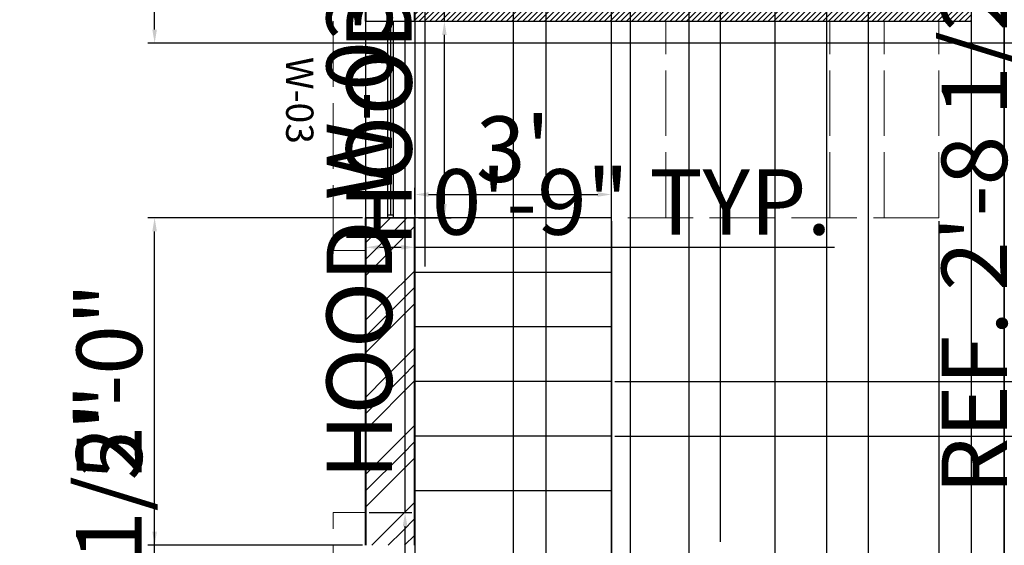
# Model space of a CAD drawing. Units: inches. Extents: x 2386 to 3029, y 792 to 1465.
# Tile 5 of 12: x 2408 to 2588, y 1044 to 1140. Entities that reach past the tile are written whole.
import ezdxf

# ---------------------------------------------------------------- set-up
doc = ezdxf.new("R2010")
doc.units = ezdxf.units.IN
doc.linetypes.add('ACAD_ISO02W100', pattern=[15, 12, -3])
for name, color, linetype, lineweight in [('A-DIMS', 1, 'Continuous', 18), ('A-STAIR', 7, 'Continuous', 25), ('A-STAIR-OVHD', 7, 'ACAD_ISO02W100', 18), ('A-TEXT', 4, 'Continuous', 25), ('A-WALL-EXT', 7, 'Continuous', 40), ('A-WALL-INT', 9, 'Continuous', 30), ('A-WALL-PATT', 9, 'Continuous', 13), ('A-WINDOW', 4, 'Continuous', 25), ('A-WINDOW-OVHD', 4, 'ACAD_ISO02W100', 18)]:
    doc.layers.add(name, color=color, linetype=linetype, lineweight=lineweight)
doc.styles.get("Standard").update_dxf_attribs({"font": 'arial.ttf'})
doc.dimstyles.new('ISO-25', dxfattribs={"dimtxt": 12, "dimasz": 2.5, "dimexe": 1.25, "dimexo": 0.625, "dimtad": 1, "dimlunit": 4, "dimtxsty": 'Standard', "dimcen": 2.5, "dimadec": 0, "dimazin": 0, "dimtfac": 1, "dimtmove": 0, "dimatfit": 3, "dimfxl": 1, "dimarcsym": 0})

# ---------------------------------------------------------------- blocks, each defined once
blk = doc.blocks.new('*D18')
at = {"layer": 'A-DIMS', "color": 0, "lineweight": -2, "transparency": 16777216}
for p, q in [((2480.19, 1104.57), (2480.19, 1109.47)), ((2482.69, 1108.22), (2513.69, 1108.22)), ((2516.19, 1104.57), (2516.19, 1109.47))]:
    blk.add_line(p, q, dxfattribs=at)
at = {"layer": 'A-DIMS', "color": 0, "transparency": 16777216}
for points in [[(2482.69, 1108.64), (2482.69, 1107.81), (2480.19, 1108.22)], [(2513.69, 1108.64), (2513.69, 1107.81), (2516.19, 1108.22)]]:
    blk.add_solid(points, dxfattribs=at)
at = {"layer": 'Defpoints', "color": 0, "transparency": 16777216}
for p in [(2516.19, 1108.22), (2480.19, 1103.95), (2516.19, 1103.95)]:
    blk.add_point(p, dxfattribs=at)
at = {"layer": 'A-DIMS', "color": 0, "transparency": 16777216, "insert": (2498.19, 1114.98), "char_height": 12, "attachment_point": 5}
blk.add_mtext("3'", dxfattribs=at)
blk = doc.blocks.new('WINDOW-36IN')
for p, q in [((0, 0), (0, 36)), ((4, 36), (4, 0)), ((4, 35.5), (5, 35.5)), ((4.5, 35.5), (4.5, 0.5)), ((5, 36), (5, 0)), ((9, 36), (9, 0)), ((5, 0.5), (4, 0.5))]:
    blk.add_line(p, q)
blk = doc.blocks.new('WINDOW-HOOD-36IN')
for p, q in [((0, 0), (0, 48)), ((0, 48), (6, 48)), ((6, 0), (0, 0))]:
    blk.add_line(p, q)
blk = doc.blocks.new('*D38')
at = {"layer": 'A-DIMS', "color": 0, "lineweight": -2, "transparency": 16777216}
for p, q in [((2471.82, 1342.95), (2483.24, 1342.95)), ((2481.99, 1340.45), (2481.99, 1273.45)), ((2471.82, 1270.95), (2483.24, 1270.95)), ((2481.99, 1270.95), (2481.99, 1095.04))]:
    blk.add_line(p, q, dxfattribs=at)
at = {"layer": 'A-DIMS', "color": 0, "transparency": 16777216}
for points in [[(2481.57, 1340.45), (2482.41, 1340.45), (2481.99, 1342.95)], [(2481.57, 1273.45), (2482.41, 1273.45), (2481.99, 1270.95)]]:
    blk.add_solid(points, dxfattribs=at)
at = {"layer": 'Defpoints', "color": 0, "transparency": 16777216}
for p in [(2471.19, 1342.95), (2471.19, 1270.95), (2481.99, 1270.95)]:
    blk.add_point(p, dxfattribs=at)
at = {"layer": 'A-DIMS', "color": 0, "transparency": 16777216, "insert": (2475.16, 1181.74), "char_height": 12, "attachment_point": 5, "rotation": 90}
blk.add_mtext('HOOD W-01 6\'-0" TYP.', dxfattribs=at)
blk = doc.blocks.new('*D44')
at = {"layer": 'A-DIMS', "color": 0, "lineweight": -2, "transparency": 16777216}
for p, q in [((2485.59, 1139.95), (2485.59, 1262.04)), ((2480.82, 1139.95), (2486.84, 1139.95)), ((2485.59, 1106.45), (2485.59, 1137.45)), ((2480.82, 1103.95), (2486.84, 1103.95))]:
    blk.add_line(p, q, dxfattribs=at)
at = {"layer": 'A-DIMS', "color": 0, "transparency": 16777216}
for points in [[(2485.17, 1137.45), (2486.01, 1137.45), (2485.59, 1139.95)], [(2485.17, 1106.45), (2486.01, 1106.45), (2485.59, 1103.95)]]:
    blk.add_solid(points, dxfattribs=at)
at = {"layer": 'Defpoints', "color": 0, "transparency": 16777216}
for p in [(2480.19, 1139.95), (2485.59, 1139.95), (2480.19, 1103.95)]:
    blk.add_point(p, dxfattribs=at)
at = {"layer": 'A-DIMS', "color": 0, "transparency": 16777216, "insert": (2478.83, 1202.25), "char_height": 12, "attachment_point": 5, "rotation": 90}
blk.add_mtext('W-03 3\'-0" TYP.', dxfattribs=at)
blk = doc.blocks.new('*D45')
at = {"layer": 'A-DIMS', "color": 0, "lineweight": -2, "transparency": 16777216}
for p, q in [((2471.19, 1103.32), (2471.19, 1097.3)), ((2480.19, 1103.32), (2480.19, 1097.3)), ((2473.69, 1098.55), (2477.69, 1098.55)), ((2480.19, 1098.55), (2557.09, 1098.55))]:
    blk.add_line(p, q, dxfattribs=at)
at = {"layer": 'A-DIMS', "color": 0, "transparency": 16777216}
for points in [[(2473.69, 1098.96), (2473.69, 1098.13), (2471.19, 1098.55)], [(2477.69, 1098.96), (2477.69, 1098.13), (2480.19, 1098.55)]]:
    blk.add_solid(points, dxfattribs=at)
at = {"layer": 'Defpoints', "color": 0, "transparency": 16777216}
for p in [(2471.19, 1103.95), (2480.19, 1103.95), (2480.19, 1098.55)]:
    blk.add_point(p, dxfattribs=at)
at = {"layer": 'A-DIMS', "color": 0, "transparency": 16777216, "insert": (2519.89, 1105.3), "char_height": 12, "attachment_point": 5}
blk.add_mtext('0\'-9" TYP.', dxfattribs=at)
blk = doc.blocks.new('*D46')
at = {"layer": 'A-DIMS', "color": 0, "lineweight": -2, "transparency": 16777216}
for p, q in [((2478.39, 1049.95), (2478.39, 1225.86)), ((2471.82, 1049.95), (2479.64, 1049.95)), ((2478.39, 1004.45), (2478.39, 1047.45)), ((2471.82, 1001.95), (2479.64, 1001.95))]:
    blk.add_line(p, q, dxfattribs=at)
at = {"layer": 'A-DIMS', "color": 0, "transparency": 16777216}
for points in [[(2477.97, 1047.45), (2478.81, 1047.45), (2478.39, 1049.95)], [(2477.97, 1004.45), (2478.81, 1004.45), (2478.39, 1001.95)]]:
    blk.add_solid(points, dxfattribs=at)
at = {"layer": 'Defpoints', "color": 0, "transparency": 16777216}
for p in [(2471.19, 1049.95), (2478.39, 1049.95), (2471.19, 1001.95)]:
    blk.add_point(p, dxfattribs=at)
at = {"layer": 'A-DIMS', "color": 0, "transparency": 16777216, "insert": (2471.55, 1139.15), "char_height": 12, "attachment_point": 5, "rotation": 90}
blk.add_mtext('HOOD W-03 4\'-0" TYP.', dxfattribs=at)
blk = doc.blocks.new('*D52')
at = {"layer": 'A-DIMS', "color": 0, "lineweight": -2, "transparency": 16777216}
for p, q in [((2595.33, 1229.95), (2589.83, 1229.95)), ((2591.08, 1227.45), (2591.08, 1199.96)), ((2595.33, 1197.46), (2589.83, 1197.46)), ((2591.08, 1197.46), (2591.08, 1050.38))]:
    blk.add_line(p, q, dxfattribs=at)
at = {"layer": 'A-DIMS', "color": 0, "transparency": 16777216}
for points in [[(2590.67, 1227.45), (2591.5, 1227.45), (2591.08, 1229.95)], [(2590.67, 1199.96), (2591.5, 1199.96), (2591.08, 1197.46)]]:
    blk.add_solid(points, dxfattribs=at)
at = {"layer": 'Defpoints', "color": 0, "transparency": 16777216}
for p in [(2595.96, 1229.95), (2591.08, 1197.46), (2595.96, 1197.46)]:
    blk.add_point(p, dxfattribs=at)
at = {"layer": 'A-DIMS', "color": 0, "transparency": 16777216, "insert": (2584.25, 1122.67), "char_height": 12, "attachment_point": 5, "rotation": 90}
blk.add_mtext('REF. 2\'-8 1/2" TYP.', dxfattribs=at)
blk = doc.blocks.new('*D57')
at = {"layer": 'A-DIMS', "color": 0, "lineweight": -2, "transparency": 16777216}
for p, q in [((2546.19, 1008.57), (2546.19, 1427.9)), ((2582.19, 1008.57), (2582.19, 1427.9)), ((2548.69, 1426.65), (2579.69, 1426.65))]:
    blk.add_line(p, q, dxfattribs=at)
at = {"layer": 'A-DIMS', "color": 0, "transparency": 16777216}
for points in [[(2548.69, 1427.06), (2548.69, 1426.23), (2546.19, 1426.65)], [(2579.69, 1427.06), (2579.69, 1426.23), (2582.19, 1426.65)]]:
    blk.add_solid(points, dxfattribs=at)
at = {"layer": 'Defpoints', "color": 0, "transparency": 16777216}
for p in [(2582.19, 1426.65), (2546.19, 1007.95), (2582.19, 1007.95)]:
    blk.add_point(p, dxfattribs=at)
at = {"layer": 'A-DIMS', "color": 0, "transparency": 16777216, "insert": (2564.19, 1433.4), "char_height": 12, "attachment_point": 5}
blk.add_mtext('3\'-0"', dxfattribs=at)
blk = doc.blocks.new('*D62')
at = {"layer": 'A-DIMS', "color": 0, "lineweight": -2, "transparency": 16777216}
for p, q in [((2432.49, 1007.95), (2432.49, 1072.04)), ((2470.57, 1007.95), (2431.24, 1007.95)), ((2432.49, 955.95), (2432.49, 1005.45)), ((2470.57, 953.45), (2431.24, 953.45))]:
    blk.add_line(p, q, dxfattribs=at)
at = {"layer": 'A-DIMS', "color": 0, "transparency": 16777216}
for points in [[(2432.07, 1005.45), (2432.91, 1005.45), (2432.49, 1007.95)], [(2432.07, 955.95), (2432.91, 955.95), (2432.49, 953.45)]]:
    blk.add_solid(points, dxfattribs=at)
at = {"layer": 'Defpoints', "color": 0, "transparency": 16777216}
for p in [(2432.49, 1007.95), (2471.19, 1007.95), (2471.19, 953.45)]:
    blk.add_point(p, dxfattribs=at)
at = {"layer": 'A-DIMS', "color": 0, "transparency": 16777216, "insert": (2425.66, 1041.24), "char_height": 12, "attachment_point": 5, "rotation": 90}
blk.add_mtext('4\'-6 1/2"', dxfattribs=at)
blk = doc.blocks.new('*D63')
at = {"layer": 'A-DIMS', "color": 0, "lineweight": -2, "transparency": 16777216}
for p, q in [((2470.57, 1103.95), (2431.24, 1103.95)), ((2432.49, 1046.45), (2432.49, 1101.45)), ((2470.57, 1043.95), (2431.24, 1043.95))]:
    blk.add_line(p, q, dxfattribs=at)
at = {"layer": 'A-DIMS', "color": 0, "transparency": 16777216}
for points in [[(2432.07, 1101.45), (2432.91, 1101.45), (2432.49, 1103.95)], [(2432.07, 1046.45), (2432.91, 1046.45), (2432.49, 1043.95)]]:
    blk.add_solid(points, dxfattribs=at)
at = {"layer": 'Defpoints', "color": 0, "transparency": 16777216}
for p in [(2432.49, 1103.95), (2471.19, 1103.95), (2471.19, 1043.95)]:
    blk.add_point(p, dxfattribs=at)
at = {"layer": 'A-DIMS', "color": 0, "transparency": 16777216, "insert": (2425.74, 1073.95), "char_height": 12, "attachment_point": 5, "rotation": 90}
blk.add_mtext('5\'-0"', dxfattribs=at)
blk = doc.blocks.new('*D73')
at = {"layer": 'A-DIMS', "color": 0, "lineweight": -2, "transparency": 16777216}
for p, q in [((2519.68, 889.97), (2519.68, 1427.9)), ((2555.68, 889.97), (2555.68, 1427.9)), ((2522.18, 1426.65), (2553.18, 1426.65))]:
    blk.add_line(p, q, dxfattribs=at)
at = {"layer": 'A-DIMS', "color": 0, "transparency": 16777216}
for points in [[(2522.18, 1427.06), (2522.18, 1426.23), (2519.68, 1426.65)], [(2553.18, 1427.06), (2553.18, 1426.23), (2555.68, 1426.65)]]:
    blk.add_solid(points, dxfattribs=at)
at = {"layer": 'Defpoints', "color": 0, "transparency": 16777216}
for p in [(2555.68, 1426.65), (2519.68, 889.35), (2555.68, 889.35)]:
    blk.add_point(p, dxfattribs=at)
at = {"layer": 'A-DIMS', "color": 0, "transparency": 16777216, "insert": (2537.68, 1433.4), "char_height": 12, "attachment_point": 5}
blk.add_mtext('3\'-0"', dxfattribs=at)
blk = doc.blocks.new('*D76')
at = {"layer": 'A-DIMS', "color": 0, "lineweight": -2, "transparency": 16777216}
for p, q in [((2480.19, 1174.77), (2480.19, 808)), ((2498.19, 1174.77), (2498.19, 808)), ((2482.69, 809.25), (2495.69, 809.25)), ((2498.19, 809.25), (2532.71, 809.25))]:
    blk.add_line(p, q, dxfattribs=at)
at = {"layer": 'A-DIMS', "color": 0, "transparency": 16777216}
for points in [[(2482.69, 809.66), (2482.69, 808.83), (2480.19, 809.25)], [(2495.69, 809.66), (2495.69, 808.83), (2498.19, 809.25)]]:
    blk.add_solid(points, dxfattribs=at)
at = {"layer": 'Defpoints', "color": 0, "transparency": 16777216}
for p in [(2480.19, 1175.39), (2498.19, 1175.39), (2498.19, 809.25)]:
    blk.add_point(p, dxfattribs=at)
at = {"layer": 'A-DIMS', "color": 0, "transparency": 16777216, "insert": (2516.7, 816), "char_height": 12, "attachment_point": 5}
blk.add_mtext('1\'-6"', dxfattribs=at)
blk = doc.blocks.new('*D77')
at = {"layer": 'A-DIMS', "color": 0, "lineweight": -2, "transparency": 16777216}
for p, q in [((2516.19, 1103.32), (2516.19, 808)), ((2576.19, 1103.32), (2576.19, 808)), ((2518.69, 809.25), (2573.69, 809.25))]:
    blk.add_line(p, q, dxfattribs=at)
at = {"layer": 'A-DIMS', "color": 0, "transparency": 16777216}
for points in [[(2518.69, 809.66), (2518.69, 808.83), (2516.19, 809.25)], [(2573.69, 809.66), (2573.69, 808.83), (2576.19, 809.25)]]:
    blk.add_solid(points, dxfattribs=at)
at = {"layer": 'Defpoints', "color": 0, "transparency": 16777216}
for p in [(2516.19, 1103.95), (2576.19, 1103.95), (2576.19, 809.25)]:
    blk.add_point(p, dxfattribs=at)
at = {"layer": 'A-DIMS', "color": 0, "transparency": 16777216, "insert": (2546.19, 816), "char_height": 12, "attachment_point": 5}
blk.add_mtext('5\'-0"', dxfattribs=at)
blk = doc.blocks.new('*D78')
at = {"layer": 'A-DIMS', "color": 0, "lineweight": -2, "transparency": 16777216}
for p, q in [((2516.19, 1054.57), (2516.19, 1427.9)), ((2536.19, 1044.57), (2536.19, 1427.9)), ((2518.69, 1426.65), (2533.69, 1426.65)), ((2536.19, 1426.65), (2570.71, 1426.65))]:
    blk.add_line(p, q, dxfattribs=at)
at = {"layer": 'A-DIMS', "color": 0, "transparency": 16777216}
for points in [[(2518.69, 1427.06), (2518.69, 1426.23), (2516.19, 1426.65)], [(2533.69, 1427.06), (2533.69, 1426.23), (2536.19, 1426.65)]]:
    blk.add_solid(points, dxfattribs=at)
at = {"layer": 'Defpoints', "color": 0, "transparency": 16777216}
for p in [(2536.19, 1426.65), (2516.19, 1053.95), (2536.19, 1043.95)]:
    blk.add_point(p, dxfattribs=at)
at = {"layer": 'A-DIMS', "color": 0, "transparency": 16777216, "insert": (2554.7, 1433.4), "char_height": 12, "attachment_point": 5}
blk.add_mtext('1\'-8"', dxfattribs=at)
blk = doc.blocks.new('*D79')
at = {"layer": 'A-DIMS', "color": 0, "lineweight": -2, "transparency": 16777216}
for p, q in [((2929.89, 1073.95), (2929.89, 1118.92)), ((2516.82, 1073.95), (2931.14, 1073.95)), ((2929.89, 1066.45), (2929.89, 1071.45)), ((2516.82, 1063.95), (2931.14, 1063.95))]:
    blk.add_line(p, q, dxfattribs=at)
at = {"layer": 'A-DIMS', "color": 0, "transparency": 16777216}
for points in [[(2929.47, 1071.45), (2930.31, 1071.45), (2929.89, 1073.95)], [(2929.47, 1066.45), (2930.31, 1066.45), (2929.89, 1063.95)]]:
    blk.add_solid(points, dxfattribs=at)
at = {"layer": 'Defpoints', "color": 0, "transparency": 16777216}
for p in [(2516.19, 1073.95), (2929.89, 1073.95), (2516.19, 1063.95)]:
    blk.add_point(p, dxfattribs=at)
at = {"layer": 'A-DIMS', "color": 0, "transparency": 16777216, "insert": (2923.14, 1097.68), "char_height": 12, "attachment_point": 5, "rotation": 90}
blk.add_mtext('0\'-10"', dxfattribs=at)
blk = doc.blocks.new('*D81')
at = {"layer": 'A-DIMS', "color": 0, "lineweight": -2, "transparency": 16777216}
for p, q in [((2432.49, 1153.95), (2432.49, 1188.47)), ((2809.57, 1153.95), (2431.24, 1153.95)), ((2432.49, 1138.45), (2432.49, 1151.45)), ((2809.57, 1135.95), (2431.24, 1135.95))]:
    blk.add_line(p, q, dxfattribs=at)
at = {"layer": 'A-DIMS', "color": 0, "transparency": 16777216}
for points in [[(2432.07, 1151.45), (2432.91, 1151.45), (2432.49, 1153.95)], [(2432.07, 1138.45), (2432.91, 1138.45), (2432.49, 1135.95)]]:
    blk.add_solid(points, dxfattribs=at)
at = {"layer": 'Defpoints', "color": 0, "transparency": 16777216}
for p in [(2432.49, 1153.95), (2810.19, 1153.95), (2810.19, 1135.95)]:
    blk.add_point(p, dxfattribs=at)
at = {"layer": 'A-DIMS', "color": 0, "transparency": 16777216, "insert": (2425.74, 1172.46), "char_height": 12, "attachment_point": 5, "rotation": 90}
blk.add_mtext('1\'-6"', dxfattribs=at)
blk = doc.blocks.new('*D94')
at = {"layer": 'A-DIMS', "color": 0, "lineweight": -2, "transparency": 16777216}
for p, q in [((2504.19, 1205.32), (2504.19, 808)), ((2588.19, 1205.32), (2588.19, 808)), ((2506.69, 809.25), (2585.69, 809.25))]:
    blk.add_line(p, q, dxfattribs=at)
at = {"layer": 'A-DIMS', "color": 0, "transparency": 16777216}
for points in [[(2506.69, 809.66), (2506.69, 808.83), (2504.19, 809.25)], [(2585.69, 809.66), (2585.69, 808.83), (2588.19, 809.25)]]:
    blk.add_solid(points, dxfattribs=at)
at = {"layer": 'Defpoints', "color": 0, "transparency": 16777216}
for p in [(2504.19, 1205.95), (2588.19, 1205.95), (2588.19, 809.25)]:
    blk.add_point(p, dxfattribs=at)
at = {"layer": 'A-DIMS', "color": 0, "transparency": 16777216, "insert": (2546.19, 816), "char_height": 12, "attachment_point": 5}
blk.add_mtext('7\'-0"', dxfattribs=at)
blk = doc.blocks.new('*D96')
at = {"layer": 'A-DIMS', "color": 0, "lineweight": -2, "transparency": 16777216}
for p, q in [((2516.19, 893.57), (2516.19, 1427.9)), ((2588.19, 893.57), (2588.19, 1427.9)), ((2518.69, 1426.65), (2585.69, 1426.65))]:
    blk.add_line(p, q, dxfattribs=at)
at = {"layer": 'A-DIMS', "color": 0, "transparency": 16777216}
for points in [[(2518.69, 1427.06), (2518.69, 1426.23), (2516.19, 1426.65)], [(2585.69, 1427.06), (2585.69, 1426.23), (2588.19, 1426.65)]]:
    blk.add_solid(points, dxfattribs=at)
at = {"layer": 'Defpoints', "color": 0, "transparency": 16777216}
for p in [(2588.19, 1426.65), (2516.19, 892.95), (2588.19, 892.95)]:
    blk.add_point(p, dxfattribs=at)
at = {"layer": 'A-DIMS', "color": 0, "transparency": 16777216, "insert": (2552.19, 1433.4), "char_height": 12, "attachment_point": 5}
blk.add_mtext('6\'-0"', dxfattribs=at)
blk = doc.blocks.new('*D99')
at = {"layer": 'A-DIMS', "color": 0, "lineweight": -2, "transparency": 16777216}
for p, q in [((2530.41, 1210.29), (2530.41, 808)), ((2563.26, 1210.63), (2563.26, 808)), ((2532.91, 809.25), (2560.76, 809.25)), ((2563.26, 809.25), (2599.11, 809.25))]:
    blk.add_line(p, q, dxfattribs=at)
at = {"layer": 'A-DIMS', "color": 0, "transparency": 16777216}
for points in [[(2532.91, 809.66), (2532.91, 808.83), (2530.41, 809.25)], [(2560.76, 809.66), (2560.76, 808.83), (2563.26, 809.25)]]:
    blk.add_solid(points, dxfattribs=at)
at = {"layer": 'Defpoints', "color": 0, "transparency": 16777216}
for p in [(2530.41, 1210.91), (2563.26, 1211.26), (2563.26, 809.25)]:
    blk.add_point(p, dxfattribs=at)
at = {"layer": 'A-DIMS', "color": 0, "transparency": 16777216, "insert": (2582.43, 816), "char_height": 12, "attachment_point": 5}
blk.add_mtext('2\'-9"', dxfattribs=at)

msp = doc.modelspace()

# ---------------------------------------------------------------- hatches: boundary and pattern name
at = {"layer": 'A-WALL-PATT'}
h = msp.add_hatch(dxfattribs=at)
h.set_pattern_fill('GOST_GROUND', color=256)
h.paths.add_polyline_path([(2480.19, 1276.948), (2471.19, 1276.948), (2471.19, 1211.948), (2480.19, 1211.948)])
h.paths.add_polyline_path([(2480.19, 1378.948), (2510.19, 1378.948), (2510.19, 1378.969), (2523.779, 1378.969), (2580.602, 1378.959), (2580.602, 1378.969), (2594.19, 1378.969), (2642.19, 1378.948), (2642.19, 1387.948), (2471.19, 1387.948), (2471.19, 1336.948), (2480.19, 1336.948)])
h.paths.add_polyline_path([(2891.19, 1387.948), (2666.19, 1387.948), (2666.19, 1378.948), (2882.19, 1378.948), (2882.19, 1355.948), (2891.19, 1355.948)])
h.paths.add_polyline_path([(2891.19, 1331.948), (2882.19, 1331.948), (2882.19, 1331.449), (2882.19, 1261.948), (2891.19, 1261.948)])
h.paths.add_polyline_path([(2891.19, 1201.948), (2882.19, 1201.948), (2882.19, 1189.948), (2882.19, 1159.948), (2882.19, 1117.948), (2891.19, 1117.948)])
h.paths.add_polyline_path([(2891.19, 1057.948), (2882.19, 1057.948), (2882.19, 856.948), (2882.19, 847.948), (2891.19, 847.948)])
h.paths.add_polyline_path([(2594.19, 856.948), (2558.19, 856.948), (2558.19, 847.948), (2594.19, 847.948)])
h.paths.add_polyline_path([(2510.19, 856.948), (2480.19, 856.948), (2480.19, 905.448), (2471.19, 905.448), (2471.19, 847.948), (2510.19, 847.948)])
h.paths.add_polyline_path([(2480.19, 1007.948), (2471.19, 1007.948), (2471.19, 953.448), (2480.19, 953.448)])
h.paths.add_polyline_path([(2480.19, 1103.948), (2471.19, 1103.948), (2471.19, 1043.948), (2480.19, 1043.948)])
h = msp.add_hatch(dxfattribs=at)
h.set_pattern_fill('JIS_WOOD', color=256)
h.paths.add_polyline_path([(2624.19, 1229.948), (2624.19, 1145.948), (2618.19, 1145.948), (2618.19, 1140.548), (2618.19, 1139.948), (2630.19, 1139.948), (2630.19, 1240.948), (2624.19, 1240.948), (2624.19, 1234.948), (2480.19, 1234.948), (2480.19, 1229.948)])
h.paths.add_polyline_path([(2582.19, 1139.948), (2582.19, 1145.948), (2480.19, 1145.948), (2480.19, 1139.948)], flags=17)
h.paths.add_polyline_path([(2480.19, 1007.948), (2480.19, 1001.948), (2546.19, 1001.948), (2546.19, 1007.348), (2546.19, 1007.948)])
h.paths.add_polyline_path([(2594.19, 1007.948), (2582.19, 1007.948), (2582.19, 1001.948), (2588.19, 1001.948), (2588.19, 856.948), (2594.19, 856.948), (2594.19, 914.948), (2606.19, 914.948), (2606.19, 920.948), (2594.19, 920.948)])
h.paths.add_polyline_path([(2738.19, 1015.948), (2882.19, 1015.948), (2882.19, 1021.948), (2738.19, 1021.948), (2738.19, 1111.948), (2732.19, 1111.948), (2732.19, 920.948), (2720.19, 920.948), (2720.19, 914.948), (2732.19, 914.948), (2732.19, 856.948), (2738.19, 856.948)])
h.paths.add_polyline_path([(2660.19, 914.948), (2660.19, 920.948), (2648.19, 920.948), (2648.19, 914.948)])
h.paths.add_polyline_path([(2738.19, 1159.948), (2738.19, 1165.948), (2737.59, 1165.948), (2732.19, 1165.948), (2732.19, 1147.948), (2737.59, 1147.948), (2738.19, 1147.948), (2738.19, 1153.948), (2882.19, 1153.948), (2882.19, 1159.948)])
h.paths.add_polyline_path([(2732.19, 1201.948), (2738.19, 1201.948), (2738.19, 1303.948), (2774.19, 1303.948), (2774.19, 1308.948), (2768.19, 1308.948), (2768.19, 1378.948), (2762.19, 1378.948), (2762.19, 1308.948), (2726.19, 1308.948), (2726.19, 1303.948), (2732.19, 1303.948)])
h.paths.add_polyline_path([(2696.19, 1303.948), (2696.19, 1308.948), (2630.19, 1308.948), (2630.19, 1378.948), (2624.19, 1378.948), (2624.19, 1276.948), (2630.19, 1276.948), (2630.19, 1303.948)])

# ---------------------------------------------------------------- linework, layer by layer
at = {"layer": 'A-STAIR'}
for p, q in [((2516.19, 1103.948), (2471.19, 1103.948)), ((2516.19, 1007.948), (2516.19, 1103.948)), ((2516.19, 1093.948), (2480.19, 1093.948)), ((2516.19, 1083.948), (2480.19, 1083.948)), ((2516.19, 1073.948), (2480.19, 1073.948)), ((2516.19, 1063.948), (2480.19, 1063.948)), ((2516.19, 1053.948), (2480.19, 1053.948))]:
    msp.add_line(p, q, dxfattribs=at)
at = {"layer": 'A-STAIR-OVHD'}
for p, q in [((2516.19, 1103.948), (2516.19, 1139.948)), ((2526.19, 1103.948), (2526.19, 1139.948)), ((2526.19, 1103.948), (2526.19, 1139.948)), ((2536.19, 1103.948), (2536.19, 1139.948)), ((2546.19, 1103.948), (2546.19, 1139.948)), ((2556.19, 1103.948), (2556.19, 1139.948)), ((2566.19, 1103.948), (2566.19, 1139.948)), ((2576.19, 1103.948), (2576.19, 1139.948)), ((2576.19, 1103.948), (2516.19, 1103.948))]:
    msp.add_line(p, q, dxfattribs=at)
at = {"layer": 'A-WALL-EXT'}
for p, q in [((2471.19, 1139.948), (2471.19, 1163.948)), ((2480.19, 1139.948), (2480.19, 1163.948)), ((2471.19, 1043.948), (2471.19, 1103.948)), ((2480.19, 1043.948), (2480.19, 1103.948))]:
    msp.add_line(p, q, dxfattribs=at)
at = {"layer": 'A-WALL-INT'}
for p, q in [((2582.19, 1139.948), (2582.19, 1145.948)), ((2471.19, 1139.948), (2582.19, 1139.948))]:
    msp.add_line(p, q, dxfattribs=at)
at = {"layer": 'A-WINDOW'}
for p, q in [((2471.19, 1139.948), (2480.19, 1139.948)), ((2471.19, 1103.948), (2480.19, 1103.948))]:
    msp.add_line(p, q, dxfattribs=at)

# ---------------------------------------------------------------- block references
msp.add_blockref('WINDOW-36IN', (2471.19, 1103.948), dxfattribs=at)
at = {"layer": 'A-WINDOW-OVHD'}
for p in [(2465.19, 1097.948), (2465.19, 1001.948)]:
    msp.add_blockref('WINDOW-HOOD-36IN', p, dxfattribs=at)

# ---------------------------------------------------------------- texts
at = {"layer": 'A-TEXT', "insert": (2461.59, 1133.423), "char_height": 5, "attachment_point": 1, "rotation": 270}
msp.add_mtext_dynamic_manual_height_columns('W-03', width=38.22215, gutter_width=12.5, heights=[0], dxfattribs=at)

# ---------------------------------------------------------------- dimensions: what is measured, and where the dimension line sits
at = {"layer": 'A-DIMS'}
for base, p1, p2, override, picture, middle in [((2536.19, 1426.648), (2516.19, 1053.948), (2536.19, 1043.948), {"dimdec": 1, "dimlfac": 1, "dimrnd": 0, "dimzin": 1, "dimdsep": 46, "dimlunit": 4, "dimfrac": 2}, '*D78', (2554.7, 1433.4)), ((2588.19, 1426.648), (2516.19, 892.948), (2588.19, 892.948), {"dimdec": 1, "dimlfac": 1, "dimrnd": 0, "dimzin": 1, "dimdsep": 46, "dimlunit": 4, "dimfrac": 2}, '*D96', (2552.19, 1433.4)), ((2555.676, 1426.648), (2519.676, 889.348), (2555.676, 889.348), {"dimdec": 1, "dimlfac": 1, "dimrnd": 0, "dimzin": 1, "dimdsep": 46, "dimlunit": 4, "dimfrac": 2}, '*D73', (2537.676, 1433.404)), ((2582.19, 1426.648), (2546.19, 1007.948), (2582.19, 1007.948), {"dimdec": 1, "dimlfac": 1, "dimrnd": 0, "dimzin": 1, "dimdsep": 46, "dimlunit": 4, "dimfrac": 2}, '*D57', (2564.19, 1433.404)), ((2563.257, 809.248), (2530.413, 1210.915), (2563.257, 1211.257), {"dimdec": 1, "dimlfac": 1, "dimrnd": 0, "dimzin": 1, "dimdsep": 46, "dimlunit": 4, "dimfrac": 2}, '*D99', (2582.434, 816)), ((2588.19, 809.248), (2504.19, 1205.948), (2588.19, 1205.948), {"dimdec": 1, "dimlfac": 1, "dimrnd": 0, "dimzin": 1, "dimdsep": 46, "dimlunit": 4, "dimfrac": 2}, '*D94', (2546.19, 816)), ((2498.19, 809.248), (2480.19, 1175.392), (2498.19, 1175.392), {"dimdec": 1, "dimlfac": 1, "dimrnd": 0, "dimzin": 1, "dimdsep": 46, "dimlunit": 4, "dimfrac": 2}, '*D76', (2516.7, 816)), ((2516.19, 1108.224), (2480.19, 1103.948), (2516.19, 1103.948), {"dimclrd": 0, "dimclre": 0, "dimclrt": 0}, '*D18', (2498.19, 1114.98)), ((2576.19, 809.248), (2516.19, 1103.948), (2576.19, 1103.948), {"dimdec": 1, "dimlfac": 1, "dimrnd": 0, "dimzin": 1, "dimdsep": 46, "dimlunit": 4, "dimfrac": 2}, '*D77', (2546.19, 816))]:
    dim = msp.add_linear_dim(base=base, p1=p1, p2=p2, dimstyle='ISO-25', override=override, dxfattribs=at)
    dim.commit()
    dim.dimension.update_dxf_attribs({"geometry": picture, "text_midpoint": middle})
for base, p1, p2, angle, text, picture, middle in [((2481.99, 1270.948), (2471.19, 1342.948), (2471.19, 1270.948), 270, 'HOOD W-01 <> TYP.', '*D38', (2475.156, 1181.744)), ((2485.59, 1139.948), (2480.19, 1103.948), (2480.19, 1139.948), 90, 'W-03 <> TYP.', '*D44', (2478.834, 1202.246)), ((2591.083, 1197.463), (2595.956, 1229.948), (2595.956, 1197.463), 270, 'REF. <> TYP.', '*D52', (2584.253, 1122.673)), ((2478.39, 1049.948), (2471.19, 1001.948), (2471.19, 1049.948), 90, 'HOOD W-03 <> TYP.', '*D46', (2471.552, 1139.152))]:
    dim = msp.add_linear_dim(base=base, p1=p1, p2=p2, angle=angle, text=text, dimstyle='ISO-25', override={"dimdec": 1, "dimlfac": 1, "dimrnd": 0, "dimzin": 1, "dimdsep": 46, "dimlunit": 4, "dimfrac": 2}, dxfattribs=at)
    dim.commit()
    dim.dimension.update_dxf_attribs({"geometry": picture, "text_midpoint": middle})
for base, p1, p2, picture, middle in [((2432.49, 1153.948), (2810.19, 1135.948), (2810.19, 1153.948), '*D81', (2425.738, 1172.458)), ((2929.89, 1073.948), (2516.19, 1063.948), (2516.19, 1073.948), '*D79', (2923.138, 1097.684)), ((2432.49, 1103.948), (2471.19, 1043.948), (2471.19, 1103.948), '*D63', (2425.738, 1073.948)), ((2432.49, 1007.948), (2471.19, 953.448), (2471.19, 1007.948), '*D62', (2425.66, 1041.245))]:
    dim = msp.add_linear_dim(base=base, p1=p1, p2=p2, angle=90, dimstyle='ISO-25', override={"dimdec": 1, "dimlfac": 1, "dimrnd": 0, "dimzin": 1, "dimdsep": 46, "dimlunit": 4, "dimfrac": 2}, dxfattribs=at)
    dim.commit()
    dim.dimension.update_dxf_attribs({"geometry": picture, "text_midpoint": middle})
dim = msp.add_linear_dim(base=(2480.19, 1098.548), p1=(2471.19, 1103.948), p2=(2480.19, 1103.948), text='<> TYP.', dimstyle='ISO-25', override={"dimdec": 1, "dimlfac": 1, "dimrnd": 0, "dimzin": 1, "dimdsep": 46, "dimlunit": 4, "dimfrac": 2}, dxfattribs=at)
dim.commit()
dim.dimension.update_dxf_attribs({"geometry": '*D45', "text_midpoint": (2519.888, 1105.3)})

doc.saveas('drawing.dxf')
